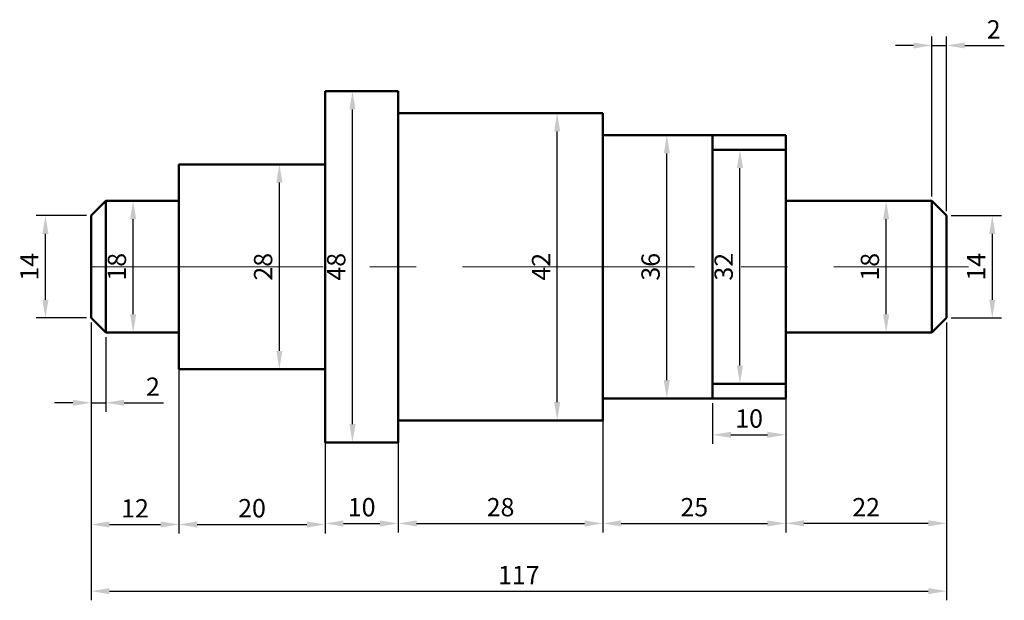
# Model space of a CAD drawing. Units: millimetres. Extents: x 2485 to 2619, y 2411 to 2490.
import ezdxf

# ---------------------------------------------------------------- set-up
doc = ezdxf.new("R2010")
doc.units = ezdxf.units.MM
doc.linetypes.add('CENTER', pattern=[50.8, 31.75, -6.35, 6.35, -6.35])
for name, color, linetype, lineweight in [('M-CNTR', 4, 'CENTER', 18), ('M-DIMS', 2, 'Continuous', 25), ('M-OUTL', 7, 'Continuous', 50)]:
    doc.layers.add(name, color=color, linetype=linetype, lineweight=lineweight)
doc.styles.get("Standard").update_dxf_attribs({"font": 'arial.ttf'})
doc.dimstyles.new('ISO-25', dxfattribs={"dimtxt": 2.5, "dimasz": 2.5, "dimexe": 1.25, "dimexo": 0.625, "dimtad": 1, "dimtxsty": 'Standard', "dimcen": 2.5, "dimadec": 0, "dimazin": 0, "dimtfac": 1, "dimtmove": 0, "dimatfit": 3, "dimfxl": 1, "dimarcsym": 0})

# ---------------------------------------------------------------- blocks, each defined once
blk = doc.blocks.new('*D1')
at = {"layer": 'Defpoints', "color": 0, "transparency": 16777216}
for p in [(2494.51, 2449.27), (2506.51, 2447.27), (2506.51, 2421.04)]:
    blk.add_point(p, dxfattribs=at)
at = {"layer": 'M-DIMS', "color": 0, "lineweight": -2, "transparency": 16777216}
for p, q in [((2494.51, 2448.64), (2494.51, 2419.79)), ((2506.51, 2446.64), (2506.51, 2419.79)), ((2497.01, 2421.04), (2504.01, 2421.04))]:
    blk.add_line(p, q, dxfattribs=at)
at = {"layer": 'M-DIMS', "color": 0, "transparency": 16777216}
for points in [[(2497.01, 2421.45), (2497.01, 2420.62), (2494.51, 2421.04)], [(2504.01, 2421.45), (2504.01, 2420.62), (2506.51, 2421.04)]]:
    blk.add_solid(points, dxfattribs=at)
at = {"layer": 'M-DIMS', "color": 0, "transparency": 16777216, "insert": (2500.51, 2422.92), "char_height": 2.5, "attachment_point": 5}
blk.add_mtext('12', dxfattribs=at)
blk = doc.blocks.new('*D2')
at = {"layer": 'Defpoints', "color": 0, "transparency": 16777216}
for p in [(2506.51, 2442.27), (2526.51, 2442.27), (2526.51, 2421.04)]:
    blk.add_point(p, dxfattribs=at)
at = {"layer": 'M-DIMS', "color": 0, "lineweight": -2, "transparency": 16777216}
for p, q in [((2506.51, 2441.64), (2506.51, 2419.79)), ((2526.51, 2441.64), (2526.51, 2419.79)), ((2509.01, 2421.04), (2524.01, 2421.04))]:
    blk.add_line(p, q, dxfattribs=at)
at = {"layer": 'M-DIMS', "color": 0, "transparency": 16777216}
for points in [[(2509.01, 2421.45), (2509.01, 2420.62), (2506.51, 2421.04)], [(2524.01, 2421.45), (2524.01, 2420.62), (2526.51, 2421.04)]]:
    blk.add_solid(points, dxfattribs=at)
at = {"layer": 'M-DIMS', "color": 0, "transparency": 16777216, "insert": (2516.51, 2422.94), "char_height": 2.5, "attachment_point": 5}
blk.add_mtext('20', dxfattribs=at)
blk = doc.blocks.new('*D3')
at = {"layer": 'Defpoints', "color": 0, "transparency": 16777216}
for p in [(2526.51, 2432.27), (2536.51, 2432.27), (2536.51, 2421.18)]:
    blk.add_point(p, dxfattribs=at)
at = {"layer": 'M-DIMS', "color": 0, "lineweight": -2, "transparency": 16777216}
for p, q in [((2526.51, 2431.64), (2526.51, 2419.93)), ((2536.51, 2431.64), (2536.51, 2419.93)), ((2529.01, 2421.18), (2534.01, 2421.18))]:
    blk.add_line(p, q, dxfattribs=at)
at = {"layer": 'M-DIMS', "color": 0, "transparency": 16777216}
for points in [[(2529.01, 2421.59), (2529.01, 2420.76), (2526.51, 2421.18)], [(2534.01, 2421.59), (2534.01, 2420.76), (2536.51, 2421.18)]]:
    blk.add_solid(points, dxfattribs=at)
at = {"layer": 'M-DIMS', "color": 0, "transparency": 16777216, "insert": (2531.51, 2423.08), "char_height": 2.5, "attachment_point": 5}
blk.add_mtext('10', dxfattribs=at)
blk = doc.blocks.new('*D4')
at = {"layer": 'Defpoints', "color": 0, "transparency": 16777216}
for p in [(2536.51, 2435.27), (2564.51, 2435.27), (2564.51, 2421.18)]:
    blk.add_point(p, dxfattribs=at)
at = {"layer": 'M-DIMS', "color": 0, "lineweight": -2, "transparency": 16777216}
for p, q in [((2536.51, 2434.64), (2536.51, 2419.93)), ((2564.51, 2434.64), (2564.51, 2419.93)), ((2539.01, 2421.18), (2562.01, 2421.18))]:
    blk.add_line(p, q, dxfattribs=at)
at = {"layer": 'M-DIMS', "color": 0, "transparency": 16777216}
for points in [[(2539.01, 2421.59), (2539.01, 2420.76), (2536.51, 2421.18)], [(2562.01, 2421.59), (2562.01, 2420.76), (2564.51, 2421.18)]]:
    blk.add_solid(points, dxfattribs=at)
at = {"layer": 'M-DIMS', "color": 0, "transparency": 16777216, "insert": (2550.51, 2423.08), "char_height": 2.5, "attachment_point": 5}
blk.add_mtext('28', dxfattribs=at)
blk = doc.blocks.new('*D5')
at = {"layer": 'Defpoints', "color": 0, "transparency": 16777216}
for p in [(2564.51, 2438.27), (2589.51, 2438.27), (2589.51, 2421.18)]:
    blk.add_point(p, dxfattribs=at)
at = {"layer": 'M-DIMS', "color": 0, "lineweight": -2, "transparency": 16777216}
for p, q in [((2564.51, 2437.64), (2564.51, 2419.93)), ((2589.51, 2437.64), (2589.51, 2419.93)), ((2567.01, 2421.18), (2587.01, 2421.18))]:
    blk.add_line(p, q, dxfattribs=at)
at = {"layer": 'M-DIMS', "color": 0, "transparency": 16777216}
for points in [[(2567.01, 2421.59), (2567.01, 2420.76), (2564.51, 2421.18)], [(2587.01, 2421.59), (2587.01, 2420.76), (2589.51, 2421.18)]]:
    blk.add_solid(points, dxfattribs=at)
at = {"layer": 'M-DIMS', "color": 0, "transparency": 16777216, "insert": (2577.01, 2423.08), "char_height": 2.5, "attachment_point": 5}
blk.add_mtext('25', dxfattribs=at)
blk = doc.blocks.new('*D6')
at = {"layer": 'Defpoints', "color": 0, "transparency": 16777216}
for p in [(2494.51, 2449.27), (2611.51, 2449.27), (2611.51, 2411.92)]:
    blk.add_point(p, dxfattribs=at)
at = {"layer": 'M-DIMS', "color": 0, "lineweight": -2, "transparency": 16777216}
for p, q in [((2494.51, 2448.64), (2494.51, 2410.67)), ((2611.51, 2448.64), (2611.51, 2410.67)), ((2497.01, 2411.92), (2609.01, 2411.92))]:
    blk.add_line(p, q, dxfattribs=at)
at = {"layer": 'M-DIMS', "color": 0, "transparency": 16777216}
for points in [[(2497.01, 2412.34), (2497.01, 2411.51), (2494.51, 2411.92)], [(2609.01, 2412.34), (2609.01, 2411.51), (2611.51, 2411.92)]]:
    blk.add_solid(points, dxfattribs=at)
at = {"layer": 'M-DIMS', "color": 0, "transparency": 16777216, "insert": (2553.01, 2413.8), "char_height": 2.5, "attachment_point": 5}
blk.add_mtext('117', dxfattribs=at)
blk = doc.blocks.new('*D7')
at = {"layer": 'Defpoints', "color": 0, "transparency": 16777216}
for p in [(2611.51, 2449.27), (2589.51, 2447.27), (2611.51, 2421.2)]:
    blk.add_point(p, dxfattribs=at)
at = {"layer": 'M-DIMS', "color": 0, "lineweight": -2, "transparency": 16777216}
for p, q in [((2611.51, 2448.64), (2611.51, 2419.95)), ((2589.51, 2446.64), (2589.51, 2419.95)), ((2592.01, 2421.2), (2609.01, 2421.2))]:
    blk.add_line(p, q, dxfattribs=at)
at = {"layer": 'M-DIMS', "color": 0, "transparency": 16777216}
for points in [[(2592.01, 2421.62), (2592.01, 2420.78), (2589.51, 2421.2)], [(2609.01, 2421.62), (2609.01, 2420.78), (2611.51, 2421.2)]]:
    blk.add_solid(points, dxfattribs=at)
at = {"layer": 'M-DIMS', "color": 0, "transparency": 16777216, "insert": (2600.51, 2423.08), "char_height": 2.5, "attachment_point": 5}
blk.add_mtext('22', dxfattribs=at)
blk = doc.blocks.new('*D8')
at = {"layer": 'Defpoints', "color": 0, "transparency": 16777216}
for p in [(2579.51, 2438.27), (2589.51, 2438.27), (2589.51, 2433.3)]:
    blk.add_point(p, dxfattribs=at)
at = {"layer": 'M-DIMS', "color": 0, "lineweight": -2, "transparency": 16777216}
for p, q in [((2579.51, 2437.64), (2579.51, 2432.05)), ((2589.51, 2437.64), (2589.51, 2432.05)), ((2582.01, 2433.3), (2587.01, 2433.3))]:
    blk.add_line(p, q, dxfattribs=at)
at = {"layer": 'M-DIMS', "color": 0, "transparency": 16777216}
for points in [[(2582.01, 2433.71), (2582.01, 2432.88), (2579.51, 2433.3)], [(2587.01, 2433.71), (2587.01, 2432.88), (2589.51, 2433.3)]]:
    blk.add_solid(points, dxfattribs=at)
at = {"layer": 'M-DIMS', "color": 0, "transparency": 16777216, "insert": (2584.51, 2435.2), "char_height": 2.5, "attachment_point": 5}
blk.add_mtext('10', dxfattribs=at)
blk = doc.blocks.new('*D9')
at = {"layer": 'Defpoints', "color": 0, "transparency": 16777216}
for p in [(2494.51, 2449.27), (2496.51, 2447.27), (2496.51, 2437.68)]:
    blk.add_point(p, dxfattribs=at)
at = {"layer": 'M-DIMS', "color": 0, "lineweight": -2, "transparency": 16777216}
for p, q in [((2494.51, 2448.64), (2494.51, 2436.43)), ((2496.51, 2446.64), (2496.51, 2436.43)), ((2492.01, 2437.68), (2489.51, 2437.68)), ((2494.51, 2437.68), (2496.51, 2437.68)), ((2499.01, 2437.68), (2504.41, 2437.68))]:
    blk.add_line(p, q, dxfattribs=at)
at = {"layer": 'M-DIMS', "color": 0, "transparency": 16777216}
for points in [[(2492.01, 2438.09), (2492.01, 2437.26), (2494.51, 2437.68)], [(2499.01, 2438.09), (2499.01, 2437.26), (2496.51, 2437.68)]]:
    blk.add_solid(points, dxfattribs=at)
at = {"layer": 'M-DIMS', "color": 0, "transparency": 16777216, "insert": (2502.96, 2439.56), "char_height": 2.5, "attachment_point": 5}
blk.add_mtext('2', dxfattribs=at)
blk = doc.blocks.new('*D10')
at = {"layer": 'Defpoints', "color": 0, "transparency": 16777216}
for p in [(2611.51, 2486.52), (2609.51, 2465.27), (2611.51, 2463.27)]:
    blk.add_point(p, dxfattribs=at)
at = {"layer": 'M-DIMS', "color": 0, "lineweight": -2, "transparency": 16777216}
for p, q in [((2609.51, 2465.89), (2609.51, 2487.77)), ((2611.51, 2463.89), (2611.51, 2487.77)), ((2607.01, 2486.52), (2604.51, 2486.52)), ((2609.51, 2486.52), (2611.51, 2486.52)), ((2614.01, 2486.52), (2619.41, 2486.52))]:
    blk.add_line(p, q, dxfattribs=at)
at = {"layer": 'M-DIMS', "color": 0, "transparency": 16777216}
for points in [[(2607.01, 2486.94), (2607.01, 2486.11), (2609.51, 2486.52)], [(2614.01, 2486.94), (2614.01, 2486.11), (2611.51, 2486.52)]]:
    blk.add_solid(points, dxfattribs=at)
at = {"layer": 'M-DIMS', "color": 0, "transparency": 16777216, "insert": (2617.96, 2488.4), "char_height": 2.5, "attachment_point": 5}
blk.add_mtext('2', dxfattribs=at)
blk = doc.blocks.new('*D11')
at = {"layer": 'Defpoints', "color": 0, "transparency": 16777216}
for p in [(2488.25, 2463.27), (2494.51, 2463.27), (2494.51, 2449.27)]:
    blk.add_point(p, dxfattribs=at)
at = {"layer": 'M-DIMS', "color": 0, "lineweight": -2, "transparency": 16777216}
for p, q in [((2493.88, 2463.27), (2487, 2463.27)), ((2488.25, 2451.77), (2488.25, 2460.77)), ((2493.88, 2449.27), (2487, 2449.27))]:
    blk.add_line(p, q, dxfattribs=at)
at = {"layer": 'M-DIMS', "color": 0, "transparency": 16777216}
for points in [[(2487.83, 2460.77), (2488.67, 2460.77), (2488.25, 2463.27)], [(2487.83, 2451.77), (2488.67, 2451.77), (2488.25, 2449.27)]]:
    blk.add_solid(points, dxfattribs=at)
at = {"layer": 'M-DIMS', "color": 0, "transparency": 16777216, "insert": (2486.37, 2456.27), "char_height": 2.5, "attachment_point": 5, "rotation": 90}
blk.add_mtext('14', dxfattribs=at)
blk = doc.blocks.new('*D12')
at = {"layer": 'Defpoints', "color": 0, "transparency": 16777216}
for p in [(2500.25, 2465.27), (2506.51, 2465.27), (2506.51, 2447.27)]:
    blk.add_point(p, dxfattribs=at)
at = {"layer": 'M-DIMS', "color": 0, "lineweight": -2, "transparency": 16777216}
for p, q in [((2505.88, 2465.27), (2499, 2465.27)), ((2500.25, 2449.77), (2500.25, 2462.77)), ((2505.88, 2447.27), (2499, 2447.27))]:
    blk.add_line(p, q, dxfattribs=at)
at = {"layer": 'M-DIMS', "color": 0, "transparency": 16777216}
for points in [[(2499.83, 2462.77), (2500.67, 2462.77), (2500.25, 2465.27)], [(2499.83, 2449.77), (2500.67, 2449.77), (2500.25, 2447.27)]]:
    blk.add_solid(points, dxfattribs=at)
at = {"layer": 'M-DIMS', "color": 0, "transparency": 16777216, "insert": (2498.35, 2456.27), "char_height": 2.5, "attachment_point": 5, "rotation": 90}
blk.add_mtext('18', dxfattribs=at)
blk = doc.blocks.new('*D13')
at = {"layer": 'Defpoints', "color": 0, "transparency": 16777216}
for p in [(2520.25, 2470.27), (2526.51, 2470.27), (2526.51, 2442.27)]:
    blk.add_point(p, dxfattribs=at)
at = {"layer": 'M-DIMS', "color": 0, "lineweight": -2, "transparency": 16777216}
for p, q in [((2525.88, 2470.27), (2519, 2470.27)), ((2520.25, 2444.77), (2520.25, 2467.77)), ((2525.88, 2442.27), (2519, 2442.27))]:
    blk.add_line(p, q, dxfattribs=at)
at = {"layer": 'M-DIMS', "color": 0, "transparency": 16777216}
for points in [[(2519.83, 2467.77), (2520.67, 2467.77), (2520.25, 2470.27)], [(2519.83, 2444.77), (2520.67, 2444.77), (2520.25, 2442.27)]]:
    blk.add_solid(points, dxfattribs=at)
at = {"layer": 'M-DIMS', "color": 0, "transparency": 16777216, "insert": (2518.35, 2456.27), "char_height": 2.5, "attachment_point": 5, "rotation": 90}
blk.add_mtext('28', dxfattribs=at)
blk = doc.blocks.new('*D14')
at = {"layer": 'Defpoints', "color": 0, "transparency": 16777216}
for p in [(2530.25, 2480.27), (2536.51, 2480.27), (2536.51, 2432.27)]:
    blk.add_point(p, dxfattribs=at)
at = {"layer": 'M-DIMS', "color": 0, "lineweight": -2, "transparency": 16777216}
for p, q in [((2535.88, 2480.27), (2529, 2480.27)), ((2530.25, 2434.77), (2530.25, 2477.77)), ((2535.88, 2432.27), (2529, 2432.27))]:
    blk.add_line(p, q, dxfattribs=at)
at = {"layer": 'M-DIMS', "color": 0, "transparency": 16777216}
for points in [[(2529.83, 2477.77), (2530.67, 2477.77), (2530.25, 2480.27)], [(2529.83, 2434.77), (2530.67, 2434.77), (2530.25, 2432.27)]]:
    blk.add_solid(points, dxfattribs=at)
at = {"layer": 'M-DIMS', "color": 0, "transparency": 16777216, "insert": (2528.35, 2456.27), "char_height": 2.5, "attachment_point": 5, "rotation": 90}
blk.add_mtext('48', dxfattribs=at)
blk = doc.blocks.new('*D15')
at = {"layer": 'Defpoints', "color": 0, "transparency": 16777216}
for p in [(2558.25, 2477.27), (2564.51, 2477.27), (2564.51, 2435.27)]:
    blk.add_point(p, dxfattribs=at)
at = {"layer": 'M-DIMS', "color": 0, "lineweight": -2, "transparency": 16777216}
for p, q in [((2563.88, 2477.27), (2557, 2477.27)), ((2558.25, 2437.77), (2558.25, 2474.77)), ((2563.88, 2435.27), (2557, 2435.27))]:
    blk.add_line(p, q, dxfattribs=at)
at = {"layer": 'M-DIMS', "color": 0, "transparency": 16777216}
for points in [[(2557.83, 2474.77), (2558.67, 2474.77), (2558.25, 2477.27)], [(2557.83, 2437.77), (2558.67, 2437.77), (2558.25, 2435.27)]]:
    blk.add_solid(points, dxfattribs=at)
at = {"layer": 'M-DIMS', "color": 0, "transparency": 16777216, "insert": (2556.37, 2456.27), "char_height": 2.5, "attachment_point": 5, "rotation": 90}
blk.add_mtext('42', dxfattribs=at)
blk = doc.blocks.new('*D16')
at = {"layer": 'Defpoints', "color": 0, "transparency": 16777216}
for p in [(2573.25, 2474.27), (2579.51, 2474.27), (2579.51, 2438.27)]:
    blk.add_point(p, dxfattribs=at)
at = {"layer": 'M-DIMS', "color": 0, "lineweight": -2, "transparency": 16777216}
for p, q in [((2578.88, 2474.27), (2572, 2474.27)), ((2573.25, 2440.77), (2573.25, 2471.77)), ((2578.88, 2438.27), (2572, 2438.27))]:
    blk.add_line(p, q, dxfattribs=at)
at = {"layer": 'M-DIMS', "color": 0, "transparency": 16777216}
for points in [[(2572.83, 2471.77), (2573.67, 2471.77), (2573.25, 2474.27)], [(2572.83, 2440.77), (2573.67, 2440.77), (2573.25, 2438.27)]]:
    blk.add_solid(points, dxfattribs=at)
at = {"layer": 'M-DIMS', "color": 0, "transparency": 16777216, "insert": (2571.35, 2456.27), "char_height": 2.5, "attachment_point": 5, "rotation": 90}
blk.add_mtext('36', dxfattribs=at)
blk = doc.blocks.new('*D17')
at = {"layer": 'Defpoints', "color": 0, "transparency": 16777216}
for p in [(2583.25, 2472.27), (2589.51, 2472.27), (2589.51, 2440.27)]:
    blk.add_point(p, dxfattribs=at)
at = {"layer": 'M-DIMS', "color": 0, "lineweight": -2, "transparency": 16777216}
for p, q in [((2588.88, 2472.27), (2582, 2472.27)), ((2583.25, 2442.77), (2583.25, 2469.77)), ((2588.88, 2440.27), (2582, 2440.27))]:
    blk.add_line(p, q, dxfattribs=at)
at = {"layer": 'M-DIMS', "color": 0, "transparency": 16777216}
for points in [[(2582.83, 2469.77), (2583.67, 2469.77), (2583.25, 2472.27)], [(2582.83, 2442.77), (2583.67, 2442.77), (2583.25, 2440.27)]]:
    blk.add_solid(points, dxfattribs=at)
at = {"layer": 'M-DIMS', "color": 0, "transparency": 16777216, "insert": (2581.35, 2456.27), "char_height": 2.5, "attachment_point": 5, "rotation": 90}
blk.add_mtext('32', dxfattribs=at)
blk = doc.blocks.new('*D18')
at = {"layer": 'Defpoints', "color": 0, "transparency": 16777216}
for p in [(2603.25, 2465.27), (2609.51, 2465.27), (2609.51, 2447.27)]:
    blk.add_point(p, dxfattribs=at)
at = {"layer": 'M-DIMS', "color": 0, "lineweight": -2, "transparency": 16777216}
for p, q in [((2608.88, 2465.27), (2602, 2465.27)), ((2603.25, 2449.77), (2603.25, 2462.77)), ((2608.88, 2447.27), (2602, 2447.27))]:
    blk.add_line(p, q, dxfattribs=at)
at = {"layer": 'M-DIMS', "color": 0, "transparency": 16777216}
for points in [[(2602.83, 2462.77), (2603.67, 2462.77), (2603.25, 2465.27)], [(2602.83, 2449.77), (2603.67, 2449.77), (2603.25, 2447.27)]]:
    blk.add_solid(points, dxfattribs=at)
at = {"layer": 'M-DIMS', "color": 0, "transparency": 16777216, "insert": (2601.35, 2456.27), "char_height": 2.5, "attachment_point": 5, "rotation": 90}
blk.add_mtext('18', dxfattribs=at)
blk = doc.blocks.new('*D19')
at = {"layer": 'Defpoints', "color": 0, "transparency": 16777216}
for p in [(2611.51, 2463.27), (2611.51, 2449.27), (2617.77, 2449.27)]:
    blk.add_point(p, dxfattribs=at)
at = {"layer": 'M-DIMS', "color": 0, "lineweight": -2, "transparency": 16777216}
for p, q in [((2612.13, 2463.27), (2619.02, 2463.27)), ((2617.77, 2460.77), (2617.77, 2451.77)), ((2612.13, 2449.27), (2619.02, 2449.27))]:
    blk.add_line(p, q, dxfattribs=at)
at = {"layer": 'M-DIMS', "color": 0, "transparency": 16777216}
for points in [[(2617.35, 2460.77), (2618.18, 2460.77), (2617.77, 2463.27)], [(2617.35, 2451.77), (2618.18, 2451.77), (2617.77, 2449.27)]]:
    blk.add_solid(points, dxfattribs=at)
at = {"layer": 'M-DIMS', "color": 0, "transparency": 16777216, "insert": (2615.89, 2456.27), "char_height": 2.5, "attachment_point": 5, "rotation": 90}
blk.add_mtext('14', dxfattribs=at)

msp = doc.modelspace()

# ---------------------------------------------------------------- linework, layer by layer
at = {"layer": 'M-CNTR'}
for q in [(2614.508, 2456.267), (2496.508, 2456.267)]:
    msp.add_line((2494.508, 2456.267), q, dxfattribs=at)
at = {"layer": 'M-OUTL'}
for p, q in [((2526.508, 2470.267), (2526.508, 2480.267)), ((2526.508, 2480.267), (2536.508, 2480.267)), ((2536.508, 2480.267), (2536.508, 2432.267)), ((2536.508, 2477.267), (2564.508, 2477.267)), ((2564.508, 2435.267), (2564.508, 2477.267)), ((2564.508, 2474.267), (2589.508, 2474.267)), ((2579.508, 2438.267), (2579.508, 2474.267)), ((2589.508, 2438.267), (2589.508, 2474.267)), ((2579.508, 2472.267), (2589.508, 2472.267)), ((2506.508, 2465.267), (2506.508, 2470.267)), ((2506.508, 2470.267), (2526.508, 2470.267)), ((2526.508, 2470.267), (2526.508, 2442.267)), ((2496.508, 2465.267), (2494.508, 2463.267)), ((2496.508, 2456.267), (2496.508, 2465.267)), ((2496.508, 2465.267), (2506.508, 2465.267)), ((2506.508, 2465.267), (2506.508, 2447.267)), ((2589.508, 2465.267), (2609.508, 2465.267)), ((2609.508, 2465.267), (2609.508, 2447.267)), ((2609.508, 2465.267), (2611.508, 2463.267)), ((2494.508, 2449.267), (2494.508, 2463.267)), ((2611.508, 2456.267), (2611.508, 2463.267)), ((2496.508, 2456.267), (2496.508, 2447.267)), ((2611.508, 2456.267), (2611.508, 2449.267)), ((2496.508, 2447.267), (2494.508, 2449.267)), ((2611.508, 2449.267), (2609.508, 2447.267)), ((2506.508, 2447.267), (2496.508, 2447.267)), ((2506.508, 2442.267), (2506.508, 2447.267)), ((2609.508, 2447.267), (2589.508, 2447.267)), ((2526.508, 2442.267), (2506.508, 2442.267)), ((2526.508, 2432.267), (2526.508, 2442.267)), ((2579.508, 2440.267), (2589.508, 2440.267)), ((2564.508, 2438.267), (2589.508, 2438.267)), ((2536.508, 2435.267), (2564.508, 2435.267)), ((2536.508, 2432.267), (2526.508, 2432.267))]:
    msp.add_line(p, q, dxfattribs=at)

# ---------------------------------------------------------------- dimensions: what is measured, and where the dimension line sits
at = {"layer": 'M-DIMS'}
for base, p1, p2, override, picture, middle in [((2611.508, 2486.525), (2609.508, 2465.267), (2611.508, 2463.267), {"dimdec": 0, "dimlfac": 1, "dimrnd": 0, "dimzin": 0, "dimdsep": 46, "dimlunit": 2}, '*D10', (2617.961, 2488.405)), ((2496.508, 2437.677), (2494.508, 2449.267), (2496.508, 2447.267), {"dimclrd": 0, "dimclre": 0, "dimclrt": 0}, '*D9', (2502.961, 2439.557)), ((2506.508, 2421.038), (2494.508, 2449.267), (2506.508, 2447.267), {"dimclrd": 0, "dimclre": 0, "dimclrt": 0}, '*D1', (2500.508, 2422.918)), ((2611.508, 2411.922), (2494.508, 2449.267), (2611.508, 2449.267), {"dimclrd": 0, "dimclre": 0, "dimclrt": 0}, '*D6', (2553.008, 2413.802)), ((2611.508, 2421.201), (2589.508, 2447.267), (2611.508, 2449.267), {"dimclrd": 0, "dimclre": 0, "dimclrt": 0}, '*D7', (2600.508, 2423.081)), ((2526.508, 2421.038), (2506.508, 2442.267), (2526.508, 2442.267), {"dimclrd": 0, "dimclre": 0, "dimclrt": 0}, '*D2', (2516.508, 2422.94)), ((2589.508, 2421.176), (2564.508, 2438.267), (2589.508, 2438.267), {"dimclrd": 0, "dimclre": 0, "dimclrt": 0}, '*D5', (2577.008, 2423.077)), ((2589.508, 2433.297), (2579.508, 2438.267), (2589.508, 2438.267), {"dimclrd": 0, "dimclre": 0, "dimclrt": 0}, '*D8', (2584.508, 2435.198)), ((2564.508, 2421.176), (2536.508, 2435.267), (2564.508, 2435.267), {"dimclrd": 0, "dimclre": 0, "dimclrt": 0}, '*D4', (2550.508, 2423.077)), ((2536.508, 2421.176), (2526.508, 2432.267), (2536.508, 2432.267), {"dimclrd": 0, "dimclre": 0, "dimclrt": 0}, '*D3', (2531.508, 2423.077))]:
    dim = msp.add_linear_dim(base=base, p1=p1, p2=p2, dimstyle='ISO-25', override=override, dxfattribs=at)
    dim.commit()
    dim.dimension.update_dxf_attribs({"geometry": picture, "text_midpoint": middle})
for base, p1, p2, angle, picture, middle in [((2530.25, 2480.267), (2536.508, 2432.267), (2536.508, 2480.267), 90, '*D14', (2528.349, 2456.267)), ((2558.25, 2477.267), (2564.508, 2435.267), (2564.508, 2477.267), 90, '*D15', (2556.37, 2456.267)), ((2573.25, 2474.267), (2579.508, 2438.267), (2579.508, 2474.267), 90, '*D16', (2571.348, 2456.267)), ((2583.25, 2472.267), (2589.508, 2440.267), (2589.508, 2472.267), 90, '*D17', (2581.348, 2456.267)), ((2520.25, 2470.267), (2526.508, 2442.267), (2526.508, 2470.267), 90, '*D13', (2518.349, 2456.267)), ((2500.25, 2465.267), (2506.508, 2447.267), (2506.508, 2465.267), 90, '*D12', (2498.349, 2456.267)), ((2603.25, 2465.267), (2609.508, 2447.267), (2609.508, 2465.267), 90, '*D18', (2601.349, 2456.267)), ((2488.25, 2463.267), (2494.508, 2449.267), (2494.508, 2463.267), 90, '*D11', (2486.37, 2456.267)), ((2617.765, 2449.267), (2611.508, 2463.267), (2611.508, 2449.267), 270, '*D19', (2615.885, 2456.267))]:
    dim = msp.add_linear_dim(base=base, p1=p1, p2=p2, angle=angle, dimstyle='ISO-25', override={"dimdec": 0, "dimlfac": 1, "dimrnd": 0, "dimzin": 0, "dimdsep": 46, "dimlunit": 2}, dxfattribs=at)
    dim.commit()
    dim.dimension.update_dxf_attribs({"geometry": picture, "text_midpoint": middle})

doc.saveas('drawing.dxf')
